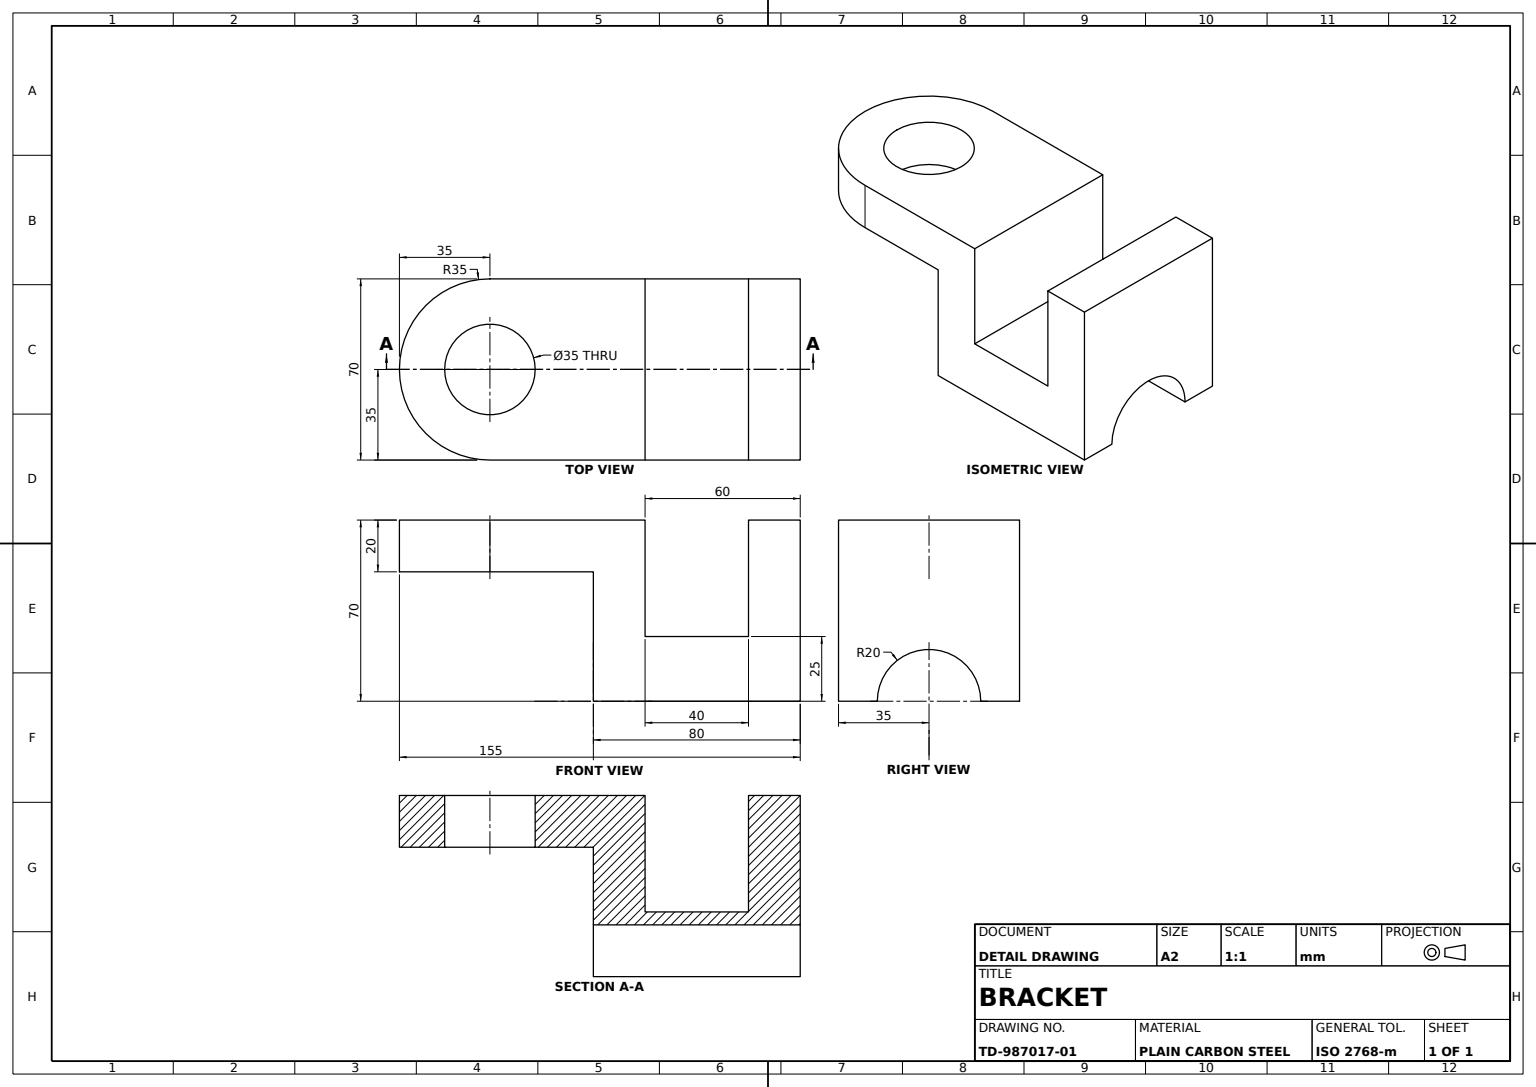
from build123d import *

# Parameters (mm, degrees)
BASE_BLOCK_SKETCH_W   = 70
BASE_BLOCK_SKETCH_H   = 70
BASE_BLOCK_DEPTH      = 20
STEP_BLOCK_SKETCH_W   = 70
STEP_BLOCK_SKETCH_H   = 40
STEP_BLOCK_DEPTH      = 25
UPPER_BLOCK_SKETCH_W  = 70
UPPER_BLOCK_SKETCH_H  = 45
UPPER_BLOCK_DEPTH     = 20
UPRIGHT_WALL_SKETCH_W = 20
UPRIGHT_WALL_SKETCH_H = 25
UPRIGHT_WALL_DEPTH    = 70
ARC_RELIEF_CUT_DEPTH  = 80
ROUNDED_LUG_DEPTH     = 20
LUG_HOLE_SKETCH_R     = 17.5
LUG_HOLE_DEPTH        = 20


with BuildPart() as part:
    # Base Block Sketch → Base Block (new body)
    with BuildSketch(Plane.XY):
        with Locations((35, -35)):
            Rectangle(BASE_BLOCK_SKETCH_W, BASE_BLOCK_SKETCH_H)
    extrude(amount=BASE_BLOCK_DEPTH)

    # Step Block Sketch → Step Block (add)
    with BuildSketch(Plane.XZ.offset(70)):
        with Locations((35, 40)):
            Rectangle(STEP_BLOCK_SKETCH_W, STEP_BLOCK_SKETCH_H)
    extrude(amount=-STEP_BLOCK_DEPTH)



with BuildPart() as body_2:
    # Upper Block Sketch → Upper Block (new body)
    with BuildSketch(Plane.XY.offset(60)):
        with Locations((35, -22.5)):
            Rectangle(UPPER_BLOCK_SKETCH_W, UPPER_BLOCK_SKETCH_H)
    extrude(amount=UPPER_BLOCK_DEPTH)


with BuildPart() as part_1:
    add(part.part)

    add(body_2.part)  # Upright Wall merges body 2
    # Upright Wall Sketch → Upright Wall (add)
    with BuildSketch(Plane.ZY):
        with Locations((70, -57.5)):
            Rectangle(UPRIGHT_WALL_SKETCH_W, UPRIGHT_WALL_SKETCH_H)
    extrude(amount=-UPRIGHT_WALL_DEPTH)

    # Arc Relief Cut Sketch → Arc Relief Cut (cut)
    with BuildSketch(Plane.XY.offset(80)):
        with BuildLine():
            Line((15, -70), (55, -70))
            ThreePointArc((55, -70), (35, -50), (15, -70))
        make_face()
    extrude(amount=-ARC_RELIEF_CUT_DEPTH, mode=Mode.SUBTRACT)

    # Rounded Lug Sketch → Rounded Lug (add)
    with BuildSketch(Plane(origin=(0, 0, 0), x_dir=(1, 0, 0), z_dir=(0, 1, 0))):
        with BuildLine():
            Line((0, -80), (70, -80))
            Line((70, -80), (70, -120))
            ThreePointArc((70, -120), (35, -155), (0, -120))
            Line((0, -120), (0, -80))
        make_face()
    extrude(amount=-ROUNDED_LUG_DEPTH)

    # Lug Hole Sketch → Lug Hole (cut)
    with BuildSketch(Plane.XZ.offset(20)):
        with Locations(Location((35, 120, 0), (0, 0, 270))):
            Circle(LUG_HOLE_SKETCH_R)
    extrude(amount=-LUG_HOLE_DEPTH, mode=Mode.SUBTRACT)


solid = part_1.part
